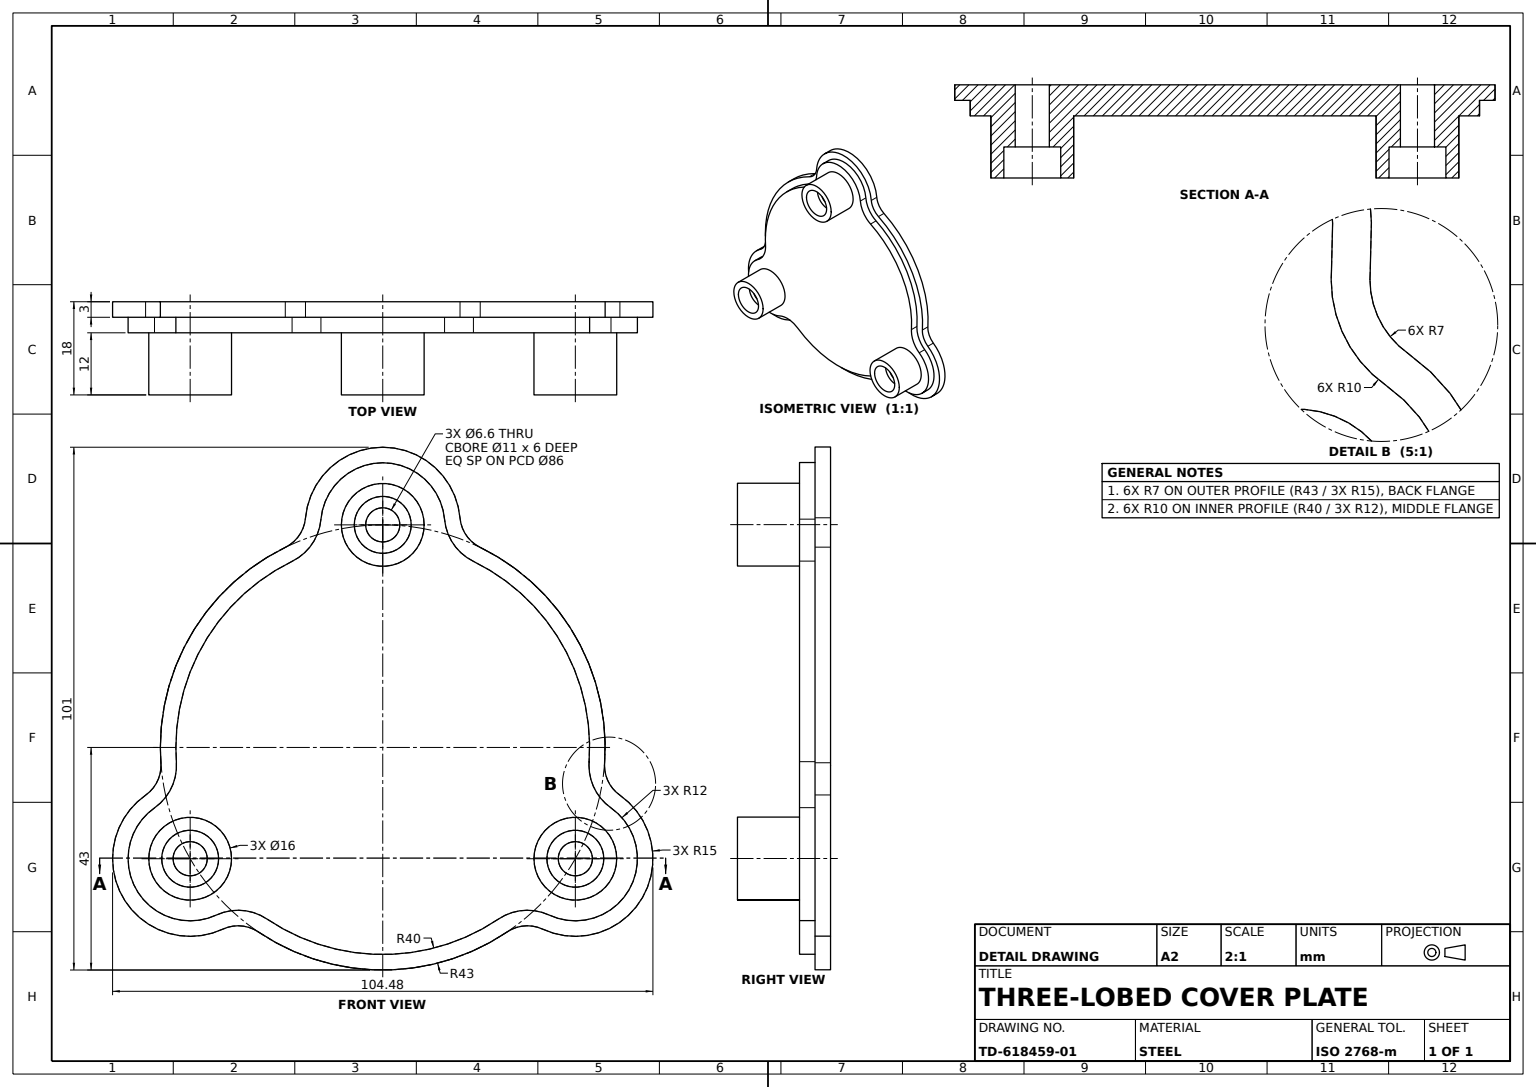
SolidWorks part; units mm, degrees
material "Plain Carbon Steel"
ref_plane "Front Plane" through (0, 0, 0) normal (0, 0, 1) x (1, 0, 0)
ref_plane "Top Plane" through (0, 0, 0) normal (0, 1, 0) x (1, 0, 0)
ref_plane "Right Plane" through (0, 0, 0) normal (1, 0, 0) x (0, 0, -1)
sketch "Base Plate Profile" plane through (0, 0, 0) normal (0, 0, 1) x (1, 0, 0)
  arc A0 (-18.8462, 38.65) -> (-42.895, -3.0038) centre (0, 0) ccw
  arc A1 (14.9415, 44.324) -> (-14.9415, 44.324) centre (0, 43) ccw
  arc A2 (30.915, -35.1017) -> (45.8564, -9.2223) centre (37.2391, -21.5) ccw
  arc A3 (-45.8564, -9.2223) -> (-30.915, -35.1017) centre (-37.2391, -21.5) ccw
  arc A4 (42.895, -3.0038) -> (18.8462, 38.65) centre (0, 0) ccw
  arc A5 (-24.0488, -35.6462) -> (24.0488, -35.6462) centre (0, 0) ccw
  arc A6 (-14.9415, 44.324) -> (-18.8462, 38.65) centre (-21.9141, 44.9419) cw
  arc A7 (-45.8564, -9.2223) -> (-42.895, -3.0038) centre (-49.8779, -3.4927) ccw
  arc A8 (-30.915, -35.1017) -> (-24.0488, -35.6462) centre (-27.9637, -41.4491) cw
  arc A9 (30.915, -35.1017) -> (24.0488, -35.6462) centre (27.9637, -41.4491) ccw
  arc A10 (45.8564, -9.2223) -> (42.895, -3.0038) centre (49.8779, -3.4927) cw
  arc A11 (14.9415, 44.324) -> (18.8462, 38.65) centre (21.9141, 44.9419) ccw
  point P17 (-27.5883, -32.9831)
  point P22 (42.3584, -7.4006)
  dimension "D1" = 3
  dimension "D2" = 43
  dimension "D3" = 15
  dimension "D6" = 7
  dimension "D7" = 7
  dimension "D4" = 37.2391
  dimension "D5" = 21.5
extrude "Base Plate 3mm" add sketch "Base Plate Profile" along normal blind 3
sketch "Raised Step Profile" plane through (0, 0, 3) normal (0, 0, 1) x (1, 0, 0)
  arc A0 (-17.5313, 35.9535) -> (-11.9532, 44.0592) centre (-21.9141, 44.9419) ccw
  arc A1 (11.9532, 44.0592) -> (-11.9532, 44.0592) centre (0, 43) ccw
  arc A2 (11.9532, 44.0592) -> (17.5313, 35.9535) centre (21.9141, 44.9419) ccw
  arc A3 (39.9023, -2.7942) -> (17.5313, 35.9535) centre (0, 0) ccw
  arc A4 (39.9023, -2.7942) -> (44.133, -11.6779) centre (49.8779, -3.4927) ccw
  arc A5 (32.1798, -32.3813) -> (44.133, -11.6779) centre (37.2391, -21.5) ccw
  arc A6 (32.1798, -32.3813) -> (22.371, -33.1593) centre (27.9637, -41.4491) ccw
  arc A7 (-22.371, -33.1593) -> (22.371, -33.1593) centre (0, 0) ccw
  arc A8 (-22.371, -33.1593) -> (-32.1798, -32.3813) centre (-27.9637, -41.4491) ccw
  arc A9 (-44.133, -11.6779) -> (-32.1798, -32.3813) centre (-37.2391, -21.5) ccw
  arc A10 (-44.133, -11.6779) -> (-39.9023, -2.7942) centre (-49.8779, -3.4927) ccw
  arc A11 (-17.5313, 35.9535) -> (-39.9023, -2.7942) centre (0, 0) ccw
  arc A12 (-18.8462, 38.65) -> (-14.9415, 44.324) centre (-21.9141, 44.9419) ccw
  arc A13 (-18.8462, 38.65) -> (-42.895, -3.0038) centre (0, 0) ccw
  arc A14 (-45.8564, -9.2223) -> (-42.895, -3.0038) centre (-49.8779, -3.4927) ccw
  arc A15 (-45.8564, -9.2223) -> (-30.915, -35.1017) centre (-37.2391, -21.5) ccw
  arc A16 (-24.0488, -35.6462) -> (-30.915, -35.1017) centre (-27.9637, -41.4491) ccw
  arc A17 (-24.0488, -35.6462) -> (24.0488, -35.6462) centre (0, 0) ccw
  arc A18 (30.915, -35.1017) -> (24.0488, -35.6462) centre (27.9637, -41.4491) ccw
  arc A19 (30.915, -35.1017) -> (45.8564, -9.2223) centre (37.2391, -21.5) ccw
  arc A20 (42.895, -3.0038) -> (45.8564, -9.2223) centre (49.8779, -3.4927) ccw
  arc A21 (42.895, -3.0038) -> (18.8462, 38.65) centre (0, 0) ccw
  arc A22 (14.9415, 44.324) -> (18.8462, 38.65) centre (21.9141, 44.9419) ccw
  arc A23 (14.9415, 44.324) -> (-14.9415, 44.324) centre (0, 43) ccw
  arc A28 (-24.0488, -35.6462) -> (-30.915, -35.1017) centre (-27.9637, -41.4491) ccw
  arc A36 (42.895, -3.0038) -> (18.8462, 38.65) centre (0, 0) ccw construction
  arc A37 (30.915, -35.1017) -> (45.8564, -9.2223) centre (37.2391, -21.5) ccw construction
  arc A38 (42.895, -3.0038) -> (45.8564, -9.2223) centre (49.8779, -3.4927) ccw construction
  arc A39 (30.915, -35.1017) -> (24.0488, -35.6462) centre (27.9637, -41.4491) ccw construction
  arc A40 (-24.0488, -35.6462) -> (24.0488, -35.6462) centre (0, 0) ccw construction
  arc A41 (-45.8564, -9.2223) -> (-30.915, -35.1017) centre (-37.2391, -21.5) ccw construction
  arc A42 (-18.8462, 38.65) -> (-42.895, -3.0038) centre (0, 0) ccw construction
  arc A43 (-45.8564, -9.2223) -> (-42.895, -3.0038) centre (-49.8779, -3.4927) ccw construction
  arc A44 (-18.8462, 38.65) -> (-14.9415, 44.324) centre (-21.9141, 44.9419) ccw construction
  arc A45 (14.9415, 44.324) -> (-14.9415, 44.324) centre (0, 43) ccw construction
  arc A46 (14.9415, 44.324) -> (18.8462, 38.65) centre (21.9141, 44.9419) ccw construction
  dimension "D1" = 0
  dimension "D2" = 3
extrude "Raised Step 3mm" add sketch "Raised Step Profile" along normal blind 3 contours A0 A11 A10 A9 A8 A7 A6 A5 A4 A3 A2 A1
sketch "Boss Profile 3xØ16" plane through (0, 0, 6) normal (0, 0, 1) x (1, 0, 0)
  circle A0 centre (0, 43) radius 8
  circle A1 centre (37.2391, -21.5) radius 8
  circle A2 centre (-37.2391, -21.5) radius 8
  dimension "D1" = 16
  dimension "D2" = 16
  dimension "D3" = 16
extrude "Bosses 3xØ16x12" add sketch "Boss Profile 3xØ16" along normal blind 12
sketch "Counterbore Profile 3xØ11" plane through (0, 0, 18) normal (0, 0, 1) x (1, 0, 0)
  circle A0 centre (0, 43) radius 5.5
  circle A1 centre (37.2391, -21.5) radius 5.5
  circle A2 centre (-37.2391, -21.5) radius 5.5
  dimension "D1" = 11
  dimension "D2" = 11
  dimension "D3" = 11
extrude "Counterbores 3xØ11x6" cut sketch "Counterbore Profile 3xØ11" against normal blind 6
sketch "Clearance Hole Profile 3xØ6.6" plane through (0, 0, 12) normal (0, 0, 1) x (1, 0, 0)
  circle A0 centre (0, 43) radius 3.3
  circle A1 centre (37.2391, -21.5) radius 3.3
  circle A2 centre (-37.2391, -21.5) radius 3.3
  dimension "D1" = 6.6
  dimension "D2" = 6.6
  dimension "D3" = 6.6
extrude "Clearance Holes 3xØ6.6 Thru" cut sketch "Clearance Hole Profile 3xØ6.6" against normal blind 146
